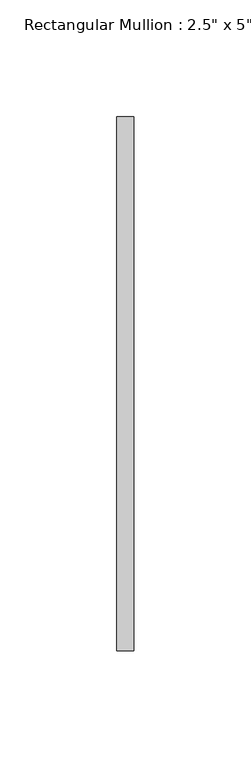
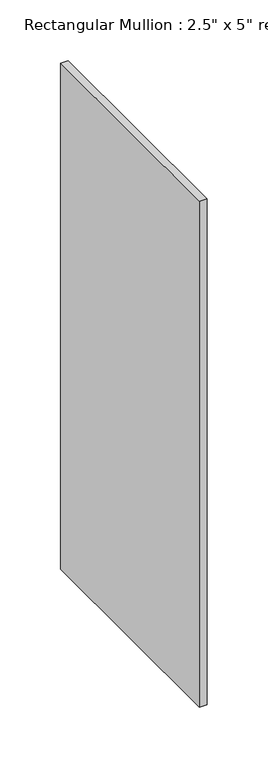
"""IFC4 building model written with IfcOpenShell, lengths in millimetres: member geometry."""

from ifc_helpers import new_model, si_unit, frame, origin, place, context, project, spatial, polyline, outline, extrude, source, transform, mapped, element, save


def member_acbd6ca0(model_context):
    return source(origin(), model_context, "Body", "SweptSolid", [
        extrude(outline(polyline([(0.0, 114.3), (0.0, -114.3), (-7.239, -114.3), (-7.239, 114.3), (0.0, 114.3)])), frame((0.0, 0.0, -508.0), z_axis=(0.0, 0.0, 1.0), x_axis=(1.0, 0.0, 0.0)), (0.0, 0.0, 1.0), 508.0),
    ])


if __name__ == "__main__":
    model = new_model("IFC4")
    model_context = context("Model", 3, world=origin())
    ifc_project = project(units=[si_unit("LENGTHUNIT", "METRE", prefix="MILLI")], contexts=[model_context])
    site = spatial("IfcSite", under=ifc_project)
    building = spatial("IfcBuilding", under=site)
    placement = place(None, origin())
    member_shape = member_acbd6ca0(model_context)
    element("IfcMember", 1, ObjectType="Rectangular Mullion : 2.5\" x 5\" rectangular", at=placement, inside=building, context=model_context, shape_type="MappedRepresentation", body=[
        mapped(member_shape, transform((0.0, 0.0, 0.0), x_axis=(1.0, 0.0, 0.0), y_axis=(0.0, 1.0, 0.0), z_axis=(0.0, 0.0, 1.0))),
    ])
    save(model, "model.ifc")

# Revit data of these elements
# Type "Rectangular Mullion : 2.5\" x 5\" rectangular"
#   built-in parameter 1007304 = 0.75 (stored number, unit not read)
#   built-in parameter 1007301 = 0.011875 (stored number, unit not read)
#   built-in parameter 1007300 = 0.011875 (stored number, unit not read)
# Element 1 (IfcMember, "Rectangular Mullion : 2.5\" x 5\" rectangular")
#   Materials on its faces: "WINDOW GLASS MATERIAL"
# Materials
#   "WINDOW GLASS MATERIAL": class "Generic", colour RGB 120 120 120, transparency 0, Cost = 0
